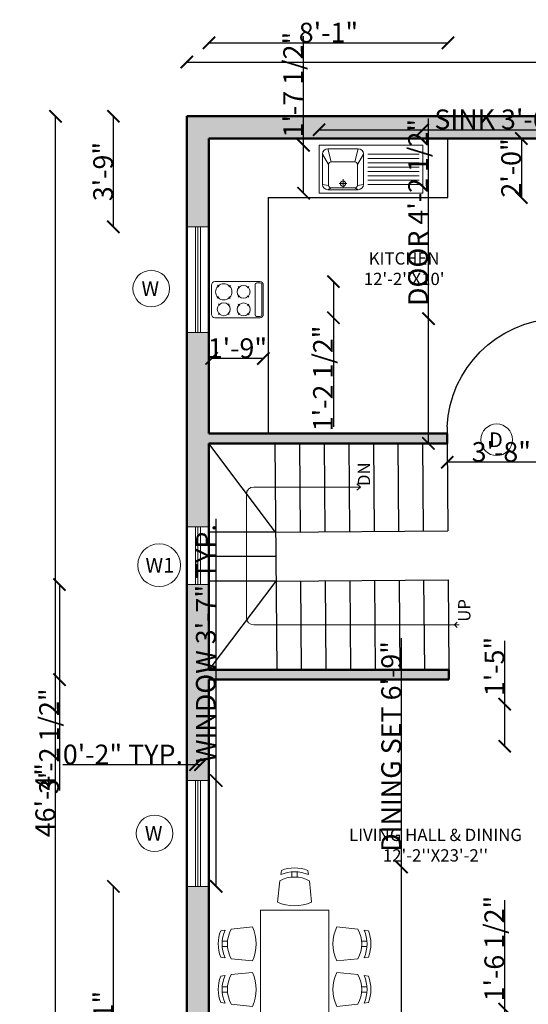
# Model space of a CAD drawing. Units: inches. Extents: x 2169 to 2662, y 1518 to 2151.
# Tile 4 of 6: x 2196 to 2403, y 1751 to 2151. Entities that reach past the tile are written whole.
import ezdxf

# ---------------------------------------------------------------- set-up
doc = ezdxf.new("R2010")
doc.units = ezdxf.units.IN
for name, color, linetype, lineweight in [('A-ANNO-DIMS', 2, 'Continuous', 18), ('A-ANNO-SYMB', 7, 'Continuous', 18), ('A-ANNO-TEXT', 7, 'Continuous', 18), ('A-AREA-IDEN', 7, 'Continuous', 18), ('A-EQPM', 8, 'Continuous', 18), ('A-FLOR-FIXT', 9, 'Continuous', 18), ('A-FURN', 8, 'Continuous', 18), ('A-WALL-PATT', 30, 'Continuous', 13), ('Doors', 240, 'Continuous', 30), ('Kitchen', 70, 'Continuous', 25), ('Steps', 50, 'Continuous', 25), ('Walls', 7, 'Continuous', 50), ('Windows', 160, 'Continuous', 18)]:
    doc.layers.add(name, color=color, linetype=linetype, lineweight=lineweight)
doc.styles.get("Standard").update_dxf_attribs({"font": 'arial.ttf'})
doc.dimstyles.get("Standard").update_dxf_attribs({"dimtxt": 8, "dimasz": 5, "dimexe": 0.18, "dimexo": 0.0625, "dimgap": 0.09, "dimtad": 1, "dimdec": 1, "dimzin": 0, "dimdsep": 46, "dimlunit": 4, "dimtxsty": 'Standard', "dimblk": 'ARCHTICK', "dimcen": 0.09, "dimse1": 1, "dimse2": 1, "dimadec": 0, "dimazin": 0, "dimtfac": 1, "dimtdec": 1, "dimtofl": 0, "dimtmove": 0, "dimatfit": 3, "dimfxl": 1, "dimtolj": 1, "dimtzin": 0, "dimarcsym": 0})

# ---------------------------------------------------------------- blocks, each defined once
blk = doc.blocks.new('_ArchTick')
at = {"color": 0, "linetype": 'ByBlock', "const_width": 0.15}
blk.add_lwpolyline([(-0.5, -0.5), (0.5, 0.5)], dxfattribs=at)
blk = doc.blocks.new('*D2')
at = {"layer": 'A-ANNO-DIMS', "color": 0, "lineweight": -2, "transparency": 16777216}
blk.add_line((2263.98, 2133.67), (2575.98, 2133.67), dxfattribs=at)
at = {"layer": 'Defpoints', "color": 0, "transparency": 16777216}
for p in [(2575.98, 2133.67), (2263.98, 2111.6), (2575.98, 2111.6)]:
    blk.add_point(p, dxfattribs=at)
at = {"layer": 'A-ANNO-DIMS', "color": 0, "lineweight": -2, "transparency": 16777216, "xscale": 5, "yscale": 5, "zscale": 5, "rotation": 180}
blk.add_blockref('_ArchTick', (2263.98, 2133.67), dxfattribs=at)
at = {"layer": 'A-ANNO-DIMS', "color": 0, "lineweight": -2, "transparency": 16777216, "xscale": 5, "yscale": 5, "zscale": 5}
blk.add_blockref('_ArchTick', (2575.98, 2133.67), dxfattribs=at)
at = {"layer": 'A-ANNO-DIMS', "color": 0, "transparency": 16777216, "insert": (2419.98, 2137.85), "char_height": 8, "attachment_point": 5}
blk.add_mtext("\\A1;26'", dxfattribs=at)
blk = doc.blocks.new('*D4')
at = {"layer": 'A-ANNO-DIMS', "color": 0, "lineweight": -2, "transparency": 16777216}
blk.add_line((2210.62, 1555.6), (2210.62, 2111.6), dxfattribs=at)
at = {"layer": 'Defpoints', "color": 0, "transparency": 16777216}
for p in [(2210.62, 2111.6), (2263.98, 2111.6), (2263.98, 1555.6)]:
    blk.add_point(p, dxfattribs=at)
at = {"layer": 'A-ANNO-DIMS', "color": 0, "lineweight": -2, "transparency": 16777216, "xscale": 5, "yscale": 5, "zscale": 5}
for p, rotation in [((2210.62, 2111.6), 90), ((2210.62, 1555.6), 270)]:
    blk.add_blockref('_ArchTick', p, dxfattribs=dict(at, rotation=rotation))
at = {"layer": 'A-ANNO-DIMS', "color": 0, "transparency": 16777216, "insert": (2206.45, 1833.6), "char_height": 8, "attachment_point": 5, "rotation": 90}
blk.add_mtext('\\A1;46\'-4"', dxfattribs=at)
blk = doc.blocks.new('table-23')
at = {"color": 0, "linetype": 'ByBlock'}
for p, q in [((-0.632, 0.469), (-0.624, 0.525)), ((-0.268, 0.469), (-0.276, 0.525)), ((-0.485, 0.506), (-0.485, 0.436)), ((-0.415, 0.506), (-0.415, 0.436)), ((-0.675, 0.107), (-0.645, 0.387)), ((-0.225, 0.107), (-0.255, 0.387)), ((-0.9, -1.492), (-0.9, 0)), ((-0.9, 0), (0, 0)), ((0, -1.492), (0, 0)), ((-1.006, -0.221), (-1.286, -0.251)), ((0.106, -0.221), (0.386, -0.251)), ((-1.368, -0.264), (-1.424, -0.273)), ((0.468, -0.264), (0.524, -0.273)), ((-1.405, -0.411), (-1.335, -0.411)), ((-1.405, -0.481), (-1.335, -0.481)), ((0.505, -0.411), (0.435, -0.411)), ((0.505, -0.481), (0.435, -0.481)), ((-1.368, -0.628), (-1.424, -0.62)), ((-1.006, -0.671), (-1.286, -0.641)), ((0.106, -0.671), (0.386, -0.641)), ((0.468, -0.628), (0.524, -0.62)), ((-1.368, -0.864), (-1.424, -0.873)), ((-1.006, -0.821), (-1.286, -0.851)), ((0.106, -0.821), (0.386, -0.851)), ((0.468, -0.864), (0.524, -0.873)), ((-1.405, -1.011), (-1.335, -1.011)), ((0.505, -1.011), (0.435, -1.011)), ((-1.405, -1.081), (-1.335, -1.081)), ((0.505, -1.081), (0.435, -1.081)), ((-1.368, -1.228), (-1.424, -1.22)), ((-1.006, -1.271), (-1.286, -1.241)), ((0.106, -1.271), (0.386, -1.241)), ((0.468, -1.228), (0.524, -1.22)), ((-0.9, -1.492), (0, -1.492)), ((-0.675, -1.599), (-0.645, -1.879)), ((-0.225, -1.599), (-0.255, -1.879)), ((-0.485, -1.998), (-0.485, -1.928)), ((-0.415, -1.998), (-0.415, -1.928)), ((-0.632, -1.961), (-0.624, -2.017)), ((-0.268, -1.961), (-0.276, -2.017))]:
    blk.add_line(p, q, dxfattribs=at)
for centre, radius, start, end in [((-0.45, 0.077), 0.48, 68.7887, 111.2113), ((-0.45, 0.032), 0.405, 61.2372, 118.7628), ((-0.45, 0.057), 0.45, 66.1344, 113.8656), ((-0.45, 0.588), 0.531, 244.9424, 295.0576), ((-0.931, -0.446), 0.405, 151.2372, 208.7628), ((-1.487, -0.446), 0.531, 334.9424, 25.0576), ((0.587, -0.446), 0.531, 154.9424, 205.0576), ((0.031, -0.446), 0.405, 331.2372, 28.7628), ((-0.977, -0.446), 0.48, 158.7887, 201.2113), ((-0.956, -0.446), 0.45, 156.1344, 203.8656), ((0.056, -0.446), 0.45, 336.1344, 23.8656), ((0.077, -0.446), 0.48, 338.7887, 21.2113), ((-0.977, -1.046), 0.48, 158.7887, 201.2113), ((-0.956, -1.046), 0.45, 156.1344, 203.8656), ((-0.931, -1.046), 0.405, 151.2372, 208.7628), ((-1.487, -1.046), 0.531, 334.9424, 25.0576), ((0.587, -1.046), 0.531, 154.9424, 205.0576), ((0.031, -1.046), 0.405, 331.2372, 28.7628), ((0.056, -1.046), 0.45, 336.1344, 23.8656), ((0.077, -1.046), 0.48, 338.7887, 21.2113), ((-0.45, -2.081), 0.531, 64.9424, 115.0576), ((-0.45, -1.524), 0.405, 241.2372, 298.7628), ((-0.45, -1.549), 0.45, 246.1344, 293.8656), ((-0.45, -1.57), 0.48, 248.7887, 291.2113)]:
    blk.add_arc(centre, radius, start, end, dxfattribs=at)
blk = doc.blocks.new('KK')
for p, q in [((0, 0.55), (0, 0)), ((1.19, 0.55), (0, 0.55)), ((0.1, 0.51), (0.14, 0.36)), ((0.45, 0.51), (0.1, 0.51)), ((0.41, 0.36), (0.45, 0.51)), ((1.19, 0), (1.19, 0.55)), ((0.11, 0.33), (0.04, 0.45)), ((0.04, 0.45), (0.04, 0.1)), ((0.14, 0.36), (0.41, 0.36)), ((0.44, 0.33), (0.51, 0.45)), ((0.51, 0.1), (0.51, 0.45)), ((0.56, 0.45), (1.15, 0.45)), ((0.56, 0.4), (1.15, 0.4)), ((0.56, 0.35), (1.15, 0.35)), ((0.11, 0.09), (0.11, 0.33)), ((0.44, 0.33), (0.44, 0.09)), ((0.56, 0.3), (1.15, 0.3)), ((0.56, 0.25), (1.15, 0.25)), ((0.275, 0.06), (0.275, 0.16)), ((0.56, 0.2), (1.15, 0.2)), ((0.56, 0.15), (1.15, 0.15)), ((0, 0), (1.19, 0)), ((0.04, 0.1), (0.11, 0.09)), ((0.14, 0.06), (0.1, 0.04)), ((0.1, 0.04), (0.45, 0.04)), ((0.41, 0.06), (0.14, 0.06)), ((0.23, 0.11), (0.32, 0.11)), ((0.41, 0.06), (0.45, 0.04)), ((0.44, 0.09), (0.51, 0.1)), ((0.56, 0.1), (1.15, 0.1))]:
    blk.add_line(p, q)
blk.add_circle((0.275, 0.11), 0.03)
for centre, radius, start, end in [((0.1, 0.45), 0.06, 90, 180), ((0.45, 0.45), 0.06, 0, 90), ((0.14, 0.33), 0.03, 90, 180), ((0.41, 0.33), 0.03, 0, 90), ((0.1, 0.1), 0.06, 180, 270), ((0.14, 0.09), 0.03, 180, 270), ((0.41, 0.09), 0.03, 270, 0), ((0.45, 0.1), 0.06, 270, 0)]:
    blk.add_arc(centre, radius, start, end)
blk = doc.blocks.new('AP0B05')
for p, q in [((35, 100), (35, 880)), ((75, 100), (75, 878.9)), ((35, 100), (35, -20)), ((815, 100), (815, -20))]:
    blk.add_line(p, q)
blk.add_lwpolyline([(35, 100), (75, 100)])
blk.add_arc((-2.4, 62.6), 818.3, 2.62122, 87.37878)
blk = doc.blocks.new('GLAZING-43IN')
for p, q in [((-21.5, 1), (21.5, 1)), ((-21.5, 0), (21.5, 0)), ((-21.5, -1), (21.5, -1))]:
    blk.add_line(p, q)
blk = doc.blocks.new('GLAZING-SHORT')
for p, q in [((-1, -11.72), (-1, 11.72)), ((0, -11.72), (0, 11.72)), ((1, -11.72), (1, 11.72))]:
    blk.add_line(p, q)
blk = doc.blocks.new('OPENING-TAG-W')
blk.add_circle((0, 0), 7.42)
blk.add_text('W', height=6).set_placement((-3.96, -3))
blk = doc.blocks.new('OPENING-TAG-D')
blk.add_circle((0, 0), 6.43)
blk.add_text('D', height=6).set_placement((-3.13, -3))
blk = doc.blocks.new('*D25')
at = {"layer": 'A-ANNO-DIMS', "color": 0, "lineweight": -2, "transparency": 16777216}
for p, q in [((2275.93, 1841.55), (2275.93, 1947.96)), ((2275.93, 1798.55), (2275.93, 1841.55))]:
    blk.add_line(p, q, dxfattribs=at)
at = {"layer": 'Defpoints', "color": 0, "transparency": 16777216}
for p in [(2269.48, 1841.55), (2275.93, 1841.55), (2269.48, 1798.55)]:
    blk.add_point(p, dxfattribs=at)
at = {"layer": 'A-ANNO-DIMS', "color": 0, "lineweight": -2, "transparency": 16777216, "xscale": 5, "yscale": 5, "zscale": 5}
for p, rotation in [((2275.93, 1841.55), 90), ((2275.93, 1798.55), 270)]:
    blk.add_blockref('_ArchTick', p, dxfattribs=dict(at, rotation=rotation))
at = {"layer": 'A-ANNO-DIMS', "color": 0, "transparency": 16777216, "insert": (2271.69, 1897.25), "char_height": 8, "attachment_point": 5, "rotation": 90}
blk.add_mtext('\\A1;WINDOW 3\'-7" TYP.', dxfattribs=at)
blk = doc.blocks.new('*D26')
at = {"layer": 'A-ANNO-DIMS', "color": 0, "lineweight": -2, "transparency": 16777216}
for p, q in [((2267.48, 1848), (2213.53, 1848)), ((2269.48, 1848), (2267.48, 1848))]:
    blk.add_line(p, q, dxfattribs=at)
at = {"layer": 'Defpoints', "color": 0, "transparency": 16777216}
for p in [(2267.48, 1848), (2267.48, 1841.55), (2269.48, 1841.55)]:
    blk.add_point(p, dxfattribs=at)
at = {"layer": 'A-ANNO-DIMS', "color": 0, "lineweight": -2, "transparency": 16777216, "xscale": 5, "yscale": 5, "zscale": 5, "rotation": 180}
blk.add_blockref('_ArchTick', (2267.48, 1848), dxfattribs=at)
at = {"layer": 'A-ANNO-DIMS', "color": 0, "lineweight": -2, "transparency": 16777216, "xscale": 5, "yscale": 5, "zscale": 5}
blk.add_blockref('_ArchTick', (2269.48, 1848), dxfattribs=at)
at = {"layer": 'A-ANNO-DIMS', "color": 0, "transparency": 16777216, "insert": (2238, 1852.17), "char_height": 8, "attachment_point": 5}
blk.add_mtext('\\A1;0\'-2" TYP.', dxfattribs=at)
blk = doc.blocks.new('*D31')
at = {"layer": 'A-ANNO-DIMS', "color": 0, "lineweight": -2, "transparency": 16777216}
for p, q in [((2362.16, 2029.35), (2362.16, 2110.67)), ((2362.16, 1978.6), (2362.16, 2029.35))]:
    blk.add_line(p, q, dxfattribs=at)
at = {"layer": 'Defpoints', "color": 0, "transparency": 16777216}
for p in [(2362.16, 2029.35), (2369.77, 2029.35), (2369.77, 1978.6)]:
    blk.add_point(p, dxfattribs=at)
at = {"layer": 'A-ANNO-DIMS', "color": 0, "lineweight": -2, "transparency": 16777216, "xscale": 5, "yscale": 5, "zscale": 5}
for p, rotation in [((2362.16, 2029.35), 90), ((2362.16, 1978.6), 270)]:
    blk.add_blockref('_ArchTick', p, dxfattribs=dict(at, rotation=rotation))
at = {"layer": 'A-ANNO-DIMS', "color": 0, "transparency": 16777216, "insert": (2357.93, 2072.51), "char_height": 8, "attachment_point": 5, "rotation": 90}
blk.add_mtext('\\A1;DOOR 4\'-2 1/2"', dxfattribs=at)
blk = doc.blocks.new('*D32')
at = {"layer": 'A-ANNO-DIMS', "color": 0, "lineweight": -2, "transparency": 16777216}
blk.add_line((2413.75, 1970.99), (2369.77, 1970.99), dxfattribs=at)
at = {"layer": 'Defpoints', "color": 0, "transparency": 16777216}
for p in [(2369.77, 1978.6), (2413.75, 1978.6), (2369.77, 1970.99)]:
    blk.add_point(p, dxfattribs=at)
at = {"layer": 'A-ANNO-DIMS', "color": 0, "lineweight": -2, "transparency": 16777216, "xscale": 5, "yscale": 5, "zscale": 5, "rotation": 180}
blk.add_blockref('_ArchTick', (2369.77, 1970.99), dxfattribs=at)
at = {"layer": 'A-ANNO-DIMS', "color": 0, "lineweight": -2, "transparency": 16777216, "xscale": 5, "yscale": 5, "zscale": 5}
blk.add_blockref('_ArchTick', (2413.75, 1970.99), dxfattribs=at)
at = {"layer": 'A-ANNO-DIMS', "color": 0, "transparency": 16777216, "insert": (2391.76, 1975.17), "char_height": 8, "attachment_point": 5}
blk.add_mtext('\\A1;3\'-8"', dxfattribs=at)
blk = doc.blocks.new('*D47')
at = {"layer": 'A-ANNO-DIMS', "color": 0, "lineweight": -2, "transparency": 16777216}
for p, q in [((2351.22, 1806.38), (2351.22, 1899.49)), ((2351.22, 1725.43), (2351.22, 1806.38))]:
    blk.add_line(p, q, dxfattribs=at)
at = {"layer": 'Defpoints', "color": 0, "transparency": 16777216}
for p in [(2339.08, 1806.38), (2351.22, 1806.38), (2339.08, 1725.43)]:
    blk.add_point(p, dxfattribs=at)
at = {"layer": 'A-ANNO-DIMS', "color": 0, "lineweight": -2, "transparency": 16777216, "xscale": 5, "yscale": 5, "zscale": 5}
for p, rotation in [((2351.22, 1806.38), 90), ((2351.22, 1725.43), 270)]:
    blk.add_blockref('_ArchTick', p, dxfattribs=dict(at, rotation=rotation))
at = {"layer": 'A-ANNO-DIMS', "color": 0, "transparency": 16777216, "insert": (2347, 1855.43), "char_height": 8, "attachment_point": 5, "rotation": 90}
blk.add_mtext('\\A1;DINING SET 6\'-9"', dxfattribs=at)
blk = doc.blocks.new('*D53')
at = {"layer": 'A-ANNO-DIMS', "color": 0, "lineweight": -2, "transparency": 16777216}
for p, q in [((2317.71, 2106.14), (2359.84, 2106.14)), ((2359.84, 2106.14), (2415.44, 2106.14))]:
    blk.add_line(p, q, dxfattribs=at)
at = {"layer": 'Defpoints', "color": 0, "transparency": 16777216}
for p in [(2359.84, 2106.14), (2317.71, 2099.82), (2359.84, 2099.82)]:
    blk.add_point(p, dxfattribs=at)
at = {"layer": 'A-ANNO-DIMS', "color": 0, "lineweight": -2, "transparency": 16777216, "xscale": 5, "yscale": 5, "zscale": 5, "rotation": 180}
blk.add_blockref('_ArchTick', (2317.71, 2106.14), dxfattribs=at)
at = {"layer": 'A-ANNO-DIMS', "color": 0, "lineweight": -2, "transparency": 16777216, "xscale": 5, "yscale": 5, "zscale": 5}
blk.add_blockref('_ArchTick', (2359.84, 2106.14), dxfattribs=at)
at = {"layer": 'A-ANNO-DIMS', "color": 0, "transparency": 16777216, "insert": (2390.14, 2110.37), "char_height": 8, "attachment_point": 5}
blk.add_mtext('\\A1;SINK 3\'-6"', dxfattribs=at)
blk = doc.blocks.new('*D54')
at = {"layer": 'A-ANNO-DIMS', "color": 0, "lineweight": -2, "transparency": 16777216}
for p, q in [((2311.39, 2099.82), (2311.39, 2144.15)), ((2311.39, 2080.34), (2311.39, 2099.82))]:
    blk.add_line(p, q, dxfattribs=at)
at = {"layer": 'Defpoints', "color": 0, "transparency": 16777216}
for p in [(2311.39, 2099.82), (2317.71, 2099.82), (2317.71, 2080.34)]:
    blk.add_point(p, dxfattribs=at)
at = {"layer": 'A-ANNO-DIMS', "color": 0, "lineweight": -2, "transparency": 16777216, "xscale": 5, "yscale": 5, "zscale": 5}
for p, rotation in [((2311.39, 2099.82), 90), ((2311.39, 2080.34), 270)]:
    blk.add_blockref('_ArchTick', p, dxfattribs=dict(at, rotation=rotation))
at = {"layer": 'A-ANNO-DIMS', "color": 0, "transparency": 16777216, "insert": (2307.16, 2124.48), "char_height": 8, "attachment_point": 5, "rotation": 90}
blk.add_mtext('\\A1;1\'-7 1/2"', dxfattribs=at)
blk = doc.blocks.new('*D59')
at = {"layer": 'A-ANNO-DIMS', "color": 0, "lineweight": -2, "transparency": 16777216}
blk.add_line((2234.13, 1689.49), (2234.13, 1798.55), dxfattribs=at)
at = {"layer": 'Defpoints', "color": 0, "transparency": 16777216}
for p in [(2234.13, 1798.55), (2263.98, 1798.55), (2263.98, 1689.49)]:
    blk.add_point(p, dxfattribs=at)
at = {"layer": 'A-ANNO-DIMS', "color": 0, "lineweight": -2, "transparency": 16777216, "xscale": 5, "yscale": 5, "zscale": 5}
for p, rotation in [((2234.13, 1798.55), 90), ((2234.13, 1689.49), 270)]:
    blk.add_blockref('_ArchTick', p, dxfattribs=dict(at, rotation=rotation))
at = {"layer": 'A-ANNO-DIMS', "color": 0, "transparency": 16777216, "insert": (2229.95, 1744.02), "char_height": 8, "attachment_point": 5, "rotation": 90}
blk.add_mtext('\\A1;9\'-1"', dxfattribs=at)
blk = doc.blocks.new('*D60')
at = {"layer": 'A-ANNO-DIMS', "color": 0, "lineweight": -2, "transparency": 16777216}
blk.add_line((2234.13, 2066.68), (2234.13, 2111.6), dxfattribs=at)
at = {"layer": 'Defpoints', "color": 0, "transparency": 16777216}
for p in [(2234.13, 2111.6), (2263.98, 2111.6), (2263.98, 2066.68)]:
    blk.add_point(p, dxfattribs=at)
at = {"layer": 'A-ANNO-DIMS', "color": 0, "lineweight": -2, "transparency": 16777216, "xscale": 5, "yscale": 5, "zscale": 5}
for p, rotation in [((2234.13, 2111.6), 90), ((2234.13, 2066.68), 270)]:
    blk.add_blockref('_ArchTick', p, dxfattribs=dict(at, rotation=rotation))
at = {"layer": 'A-ANNO-DIMS', "color": 0, "transparency": 16777216, "insert": (2229.95, 2089.14), "char_height": 8, "attachment_point": 5, "rotation": 90}
blk.add_mtext('\\A1;3\'-9"', dxfattribs=at)
blk = doc.blocks.new('*D68')
at = {"layer": 'A-ANNO-DIMS', "color": 0, "lineweight": -2, "transparency": 16777216}
blk.add_line((2272.98, 2141.45), (2370.07, 2141.45), dxfattribs=at)
at = {"layer": 'Defpoints', "color": 0, "transparency": 16777216}
for p in [(2370.07, 2141.45), (2272.98, 2102.6), (2370.07, 2102.6)]:
    blk.add_point(p, dxfattribs=at)
at = {"layer": 'A-ANNO-DIMS', "color": 0, "lineweight": -2, "transparency": 16777216, "xscale": 5, "yscale": 5, "zscale": 5, "rotation": 180}
blk.add_blockref('_ArchTick', (2272.98, 2141.45), dxfattribs=at)
at = {"layer": 'A-ANNO-DIMS', "color": 0, "lineweight": -2, "transparency": 16777216, "xscale": 5, "yscale": 5, "zscale": 5}
blk.add_blockref('_ArchTick', (2370.07, 2141.45), dxfattribs=at)
at = {"layer": 'A-ANNO-DIMS', "color": 0, "transparency": 16777216, "insert": (2321.52, 2145.63), "char_height": 8, "attachment_point": 5}
blk.add_mtext('\\A1;8\'-1"', dxfattribs=at)
blk = doc.blocks.new('*D69')
at = {"layer": 'A-ANNO-DIMS', "color": 0, "lineweight": -2, "transparency": 16777216}
blk.add_line((2399.92, 2102.6), (2399.92, 2078.6), dxfattribs=at)
at = {"layer": 'Defpoints', "color": 0, "transparency": 16777216}
for p in [(2370.07, 2102.6), (2370.07, 2078.6), (2399.92, 2078.6)]:
    blk.add_point(p, dxfattribs=at)
at = {"layer": 'A-ANNO-DIMS', "color": 0, "lineweight": -2, "transparency": 16777216, "xscale": 5, "yscale": 5, "zscale": 5}
for p, rotation in [((2399.92, 2102.6), 90), ((2399.92, 2078.6), 270)]:
    blk.add_blockref('_ArchTick', p, dxfattribs=dict(at, rotation=rotation))
at = {"layer": 'A-ANNO-DIMS', "color": 0, "transparency": 16777216, "insert": (2395.74, 2090.6), "char_height": 8, "attachment_point": 5, "rotation": 90}
blk.add_mtext('\\A1;2\'-0"', dxfattribs=at)
blk = doc.blocks.new('*D70')
at = {"layer": 'A-ANNO-DIMS', "color": 0, "lineweight": -2, "transparency": 16777216}
blk.add_line((2272.98, 1525.75), (2370.48, 1525.75), dxfattribs=at)
at = {"layer": 'Defpoints', "color": 0, "transparency": 16777216}
for p in [(2272.98, 1886.6), (2370.48, 1886.6), (2370.48, 1525.75)]:
    blk.add_point(p, dxfattribs=at)
at = {"layer": 'A-ANNO-DIMS', "color": 0, "lineweight": -2, "transparency": 16777216, "xscale": 5, "yscale": 5, "zscale": 5, "rotation": 180}
blk.add_blockref('_ArchTick', (2272.98, 1525.75), dxfattribs=at)
at = {"layer": 'A-ANNO-DIMS', "color": 0, "lineweight": -2, "transparency": 16777216, "xscale": 5, "yscale": 5, "zscale": 5}
blk.add_blockref('_ArchTick', (2370.48, 1525.75), dxfattribs=at)
at = {"layer": 'A-ANNO-DIMS', "color": 0, "transparency": 16777216, "insert": (2321.73, 1529.98), "char_height": 8, "attachment_point": 5}
blk.add_mtext('\\A1;8\'-1 1/2"', dxfattribs=at)
blk = doc.blocks.new('*D71')
at = {"layer": 'A-ANNO-DIMS', "color": 0, "lineweight": -2, "transparency": 16777216}
for p, q in [((2300.48, 1525.75), (2310.48, 1525.75)), ((2310.48, 1525.75), (2343.14, 1525.75))]:
    blk.add_line(p, q, dxfattribs=at)
at = {"layer": 'Defpoints', "color": 0, "transparency": 16777216}
for p in [(2300.48, 1886.6), (2310.48, 1886.6), (2310.48, 1525.75)]:
    blk.add_point(p, dxfattribs=at)
at = {"layer": 'A-ANNO-DIMS', "color": 0, "lineweight": -2, "transparency": 16777216, "xscale": 5, "yscale": 5, "zscale": 5, "rotation": 180}
blk.add_blockref('_ArchTick', (2300.48, 1525.75), dxfattribs=at)
at = {"layer": 'A-ANNO-DIMS', "color": 0, "lineweight": -2, "transparency": 16777216, "xscale": 5, "yscale": 5, "zscale": 5}
blk.add_blockref('_ArchTick', (2310.48, 1525.75), dxfattribs=at)
at = {"layer": 'A-ANNO-DIMS', "color": 0, "transparency": 16777216, "insert": (2329.31, 1529.93), "char_height": 8, "attachment_point": 5}
blk.add_mtext('\\A1;0\'-10"', dxfattribs=at)
blk = doc.blocks.new('*D72')
at = {"layer": 'A-ANNO-DIMS', "color": 0, "lineweight": -2, "transparency": 16777216}
blk.add_line((2624.02, 1978.6), (2624.02, 1942.6), dxfattribs=at)
at = {"layer": 'Defpoints', "color": 0, "transparency": 16777216}
for p in [(2299.77, 1978.6), (2300.05, 1942.6), (2624.02, 1942.6)]:
    blk.add_point(p, dxfattribs=at)
at = {"layer": 'A-ANNO-DIMS', "color": 0, "lineweight": -2, "transparency": 16777216, "xscale": 5, "yscale": 5, "zscale": 5}
for p, rotation in [((2624.02, 1978.6), 90), ((2624.02, 1942.6), 270)]:
    blk.add_blockref('_ArchTick', p, dxfattribs=dict(at, rotation=rotation))
at = {"layer": 'A-ANNO-DIMS', "color": 0, "transparency": 16777216, "insert": (2619.84, 1960.6), "char_height": 8, "attachment_point": 5, "rotation": 90}
blk.add_mtext('\\A1;3\'-0"', dxfattribs=at)
blk = doc.blocks.new('*D73')
at = {"layer": 'A-ANNO-DIMS', "color": 0, "lineweight": -2, "transparency": 16777216}
blk.add_line((2624.02, 1886.6), (2624.02, 1978.6), dxfattribs=at)
at = {"layer": 'Defpoints', "color": 0, "transparency": 16777216}
for p in [(2369.77, 1978.6), (2624.02, 1978.6), (2370.48, 1886.6)]:
    blk.add_point(p, dxfattribs=at)
at = {"layer": 'A-ANNO-DIMS', "color": 0, "lineweight": -2, "transparency": 16777216, "xscale": 5, "yscale": 5, "zscale": 5}
for p, rotation in [((2624.02, 1978.6), 90), ((2624.02, 1886.6), 270)]:
    blk.add_blockref('_ArchTick', p, dxfattribs=dict(at, rotation=rotation))
at = {"layer": 'A-ANNO-DIMS', "color": 0, "transparency": 16777216, "insert": (2619.84, 1932.6), "char_height": 8, "attachment_point": 5, "rotation": 90}
blk.add_mtext('\\A1;7\'-8"', dxfattribs=at)
blk = doc.blocks.new('*D74')
at = {"layer": 'A-ANNO-DIMS', "color": 0, "lineweight": -2, "transparency": 16777216}
for p, q in [((2272.98, 1525.75), (2300.48, 1525.75)), ((2300.48, 1525.75), (2345.7, 1525.75))]:
    blk.add_line(p, q, dxfattribs=at)
at = {"layer": 'Defpoints', "color": 0, "transparency": 16777216}
for p in [(2272.98, 1886.6), (2300.48, 1886.6), (2300.48, 1525.75)]:
    blk.add_point(p, dxfattribs=at)
at = {"layer": 'A-ANNO-DIMS', "color": 0, "lineweight": -2, "transparency": 16777216, "xscale": 5, "yscale": 5, "zscale": 5, "rotation": 180}
blk.add_blockref('_ArchTick', (2272.98, 1525.75), dxfattribs=at)
at = {"layer": 'A-ANNO-DIMS', "color": 0, "lineweight": -2, "transparency": 16777216, "xscale": 5, "yscale": 5, "zscale": 5}
blk.add_blockref('_ArchTick', (2300.48, 1525.75), dxfattribs=at)
at = {"layer": 'A-ANNO-DIMS', "color": 0, "transparency": 16777216, "insert": (2325.59, 1529.98), "char_height": 8, "attachment_point": 5}
blk.add_mtext('\\A1;2\'-3 1/2"', dxfattribs=at)
blk = doc.blocks.new('*D75')
at = {"layer": 'A-ANNO-DIMS', "color": 0, "lineweight": -2, "transparency": 16777216}
for p, q in [((2212.23, 1921.26), (2212.23, 1882.6)), ((2212.23, 1882.6), (2212.23, 1837.52))]:
    blk.add_line(p, q, dxfattribs=at)
at = {"layer": 'Defpoints', "color": 0, "transparency": 16777216}
for p in [(2263.98, 1921.26), (2212.23, 1882.6), (2272.98, 1882.6)]:
    blk.add_point(p, dxfattribs=at)
at = {"layer": 'A-ANNO-DIMS', "color": 0, "lineweight": -2, "transparency": 16777216, "xscale": 5, "yscale": 5, "zscale": 5}
for p, rotation in [((2212.23, 1921.26), 90), ((2212.23, 1882.6), 270)]:
    blk.add_blockref('_ArchTick', p, dxfattribs=dict(at, rotation=rotation))
at = {"layer": 'A-ANNO-DIMS', "color": 0, "transparency": 16777216, "insert": (2208, 1857.56), "char_height": 8, "attachment_point": 5, "rotation": 90}
blk.add_mtext('\\A1;3\'-2 1/2"', dxfattribs=at)
blk = doc.blocks.new('*D78')
at = {"layer": 'A-ANNO-DIMS', "color": 0, "lineweight": -2, "transparency": 16777216}
for p, q in [((2393.13, 1748.6), (2393.13, 1792.94)), ((2393.13, 1729.93), (2393.13, 1748.6))]:
    blk.add_line(p, q, dxfattribs=at)
at = {"layer": 'Defpoints', "color": 0, "transparency": 16777216}
for p in [(2393.13, 1748.6), (2422.98, 1748.6), (2422.98, 1729.93)]:
    blk.add_point(p, dxfattribs=at)
at = {"layer": 'A-ANNO-DIMS', "color": 0, "lineweight": -2, "transparency": 16777216, "xscale": 5, "yscale": 5, "zscale": 5}
for p, rotation in [((2393.13, 1748.6), 90), ((2393.13, 1729.93), 270)]:
    blk.add_blockref('_ArchTick', p, dxfattribs=dict(at, rotation=rotation))
at = {"layer": 'A-ANNO-DIMS', "color": 0, "transparency": 16777216, "insert": (2388.9, 1773.27), "char_height": 8, "attachment_point": 5, "rotation": 90}
blk.add_mtext('\\A1;1\'-6 1/2"', dxfattribs=at)
blk = doc.blocks.new('*D79')
at = {"layer": 'A-ANNO-DIMS', "color": 0, "lineweight": -2, "transparency": 16777216}
for p, q in [((2393.13, 1872.6), (2393.13, 1898.3)), ((2393.13, 1855.49), (2393.13, 1872.6))]:
    blk.add_line(p, q, dxfattribs=at)
at = {"layer": 'Defpoints', "color": 0, "transparency": 16777216}
for p in [(2393.13, 1872.6), (2422.98, 1872.6), (2422.98, 1855.49)]:
    blk.add_point(p, dxfattribs=at)
at = {"layer": 'A-ANNO-DIMS', "color": 0, "lineweight": -2, "transparency": 16777216, "xscale": 5, "yscale": 5, "zscale": 5}
for p, rotation in [((2393.13, 1872.6), 90), ((2393.13, 1855.49), 270)]:
    blk.add_blockref('_ArchTick', p, dxfattribs=dict(at, rotation=rotation))
at = {"layer": 'A-ANNO-DIMS', "color": 0, "transparency": 16777216, "insert": (2388.95, 1887.95), "char_height": 8, "attachment_point": 5, "rotation": 90}
blk.add_mtext('\\A1;1\'-5"', dxfattribs=at)
blk = doc.blocks.new('*D82')
at = {"layer": 'A-ANNO-DIMS', "color": 0, "lineweight": -2, "transparency": 16777216}
blk.add_line((2295.05, 2013.16), (2274.01, 2013.16), dxfattribs=at)
at = {"layer": 'Defpoints', "color": 0, "transparency": 16777216}
for p in [(2274.01, 2043.01), (2295.05, 2043.01), (2274.01, 2013.16)]:
    blk.add_point(p, dxfattribs=at)
at = {"layer": 'A-ANNO-DIMS', "color": 0, "lineweight": -2, "transparency": 16777216, "xscale": 5, "yscale": 5, "zscale": 5, "rotation": 180}
blk.add_blockref('_ArchTick', (2274.01, 2013.16), dxfattribs=at)
at = {"layer": 'A-ANNO-DIMS', "color": 0, "lineweight": -2, "transparency": 16777216, "xscale": 5, "yscale": 5, "zscale": 5}
blk.add_blockref('_ArchTick', (2295.05, 2013.16), dxfattribs=at)
at = {"layer": 'A-ANNO-DIMS', "color": 0, "transparency": 16777216, "insert": (2284.53, 2017.33), "char_height": 8, "attachment_point": 5}
blk.add_mtext('\\A1;1\'-9"', dxfattribs=at)
blk = doc.blocks.new('*D83')
at = {"layer": 'A-ANNO-DIMS', "color": 0, "lineweight": -2, "transparency": 16777216}
for p, q in [((2323.52, 2044.39), (2323.52, 2029.72)), ((2323.52, 2029.72), (2323.52, 1985.38))]:
    blk.add_line(p, q, dxfattribs=at)
at = {"layer": 'Defpoints', "color": 0, "transparency": 16777216}
for p in [(2293.67, 2044.39), (2293.67, 2029.72), (2323.52, 2029.72)]:
    blk.add_point(p, dxfattribs=at)
at = {"layer": 'A-ANNO-DIMS', "color": 0, "lineweight": -2, "transparency": 16777216, "xscale": 5, "yscale": 5, "zscale": 5}
for p, rotation in [((2323.52, 2044.39), 90), ((2323.52, 2029.72), 270)]:
    blk.add_blockref('_ArchTick', p, dxfattribs=dict(at, rotation=rotation))
at = {"layer": 'A-ANNO-DIMS', "color": 0, "transparency": 16777216, "insert": (2319.29, 2005.05), "char_height": 8, "attachment_point": 5, "rotation": 90}
blk.add_mtext('\\A1;1\'-2 1/2"', dxfattribs=at)

msp = doc.modelspace()

# ---------------------------------------------------------------- hatches: boundary and pattern name
at = {"layer": 'A-WALL-PATT', "transparency": 33554585}
h = msp.add_hatch(color=256, dxfattribs=at)
h.dxf.hatch_style = 1
h.paths.add_polyline_path([(2575.98, 2111.6), (2263.98, 2111.6), (2263.98, 2066.68), (2272.98, 2066.68), (2272.98, 2102.6), (2418.98, 2102.6), (2418.98, 1982.6), (2413.75, 1982.6), (2413.75, 1978.6), (2418.98, 1978.6), (2418.98, 1954.6), (2429.26, 1954.6), (2429.26, 1958.6), (2422.98, 1958.6), (2422.98, 2102.6), (2566.98, 2102.6), (2566.98, 2052.1), (2575.98, 2052.1)])
h.paths.add_polyline_path([(2575.98, 2009.1), (2566.98, 2009.1), (2566.98, 1997.84), (2566.98, 1958.6), (2467.98, 1958.6), (2467.98, 1950.67), (2471.98, 1950.67), (2471.98, 1954.6), (2566.98, 1954.6), (2566.98, 1947.83), (2575.98, 1947.83)])
h.paths.add_polyline_path([(2272.98, 2023.68), (2263.98, 2023.68), (2263.98, 1944.7), (2272.98, 1944.7), (2272.98, 1978.6), (2369.77, 1978.6), (2369.77, 1982.6), (2272.98, 1982.6)])
h.paths.add_polyline_path([(2272.98, 1882.6), (2370.48, 1882.6), (2370.48, 1886.6), (2272.98, 1886.6), (2272.98, 1921.26), (2263.98, 1921.26), (2263.98, 1841.55), (2272.98, 1841.55)])
h.paths.add_polyline_path([(2272.98, 1798.55), (2263.98, 1798.55), (2263.98, 1689.49), (2272.98, 1689.49)])
h.paths.add_polyline_path([(2272.98, 1646.49), (2263.98, 1646.49), (2263.98, 1595.6), (2281.85, 1595.6), (2281.85, 1604.6), (2272.98, 1604.6)])
h.paths.add_polyline_path([(2342.72, 1600.02), (2342.72, 1604.6), (2324.85, 1604.6), (2324.85, 1595.6), (2342.72, 1595.6)])
h.paths.add_polyline_path([(2462.45, 1604.6), (2408.92, 1604.6), (2408.92, 1595.6), (2462.45, 1595.6)])
h.paths.add_polyline_path([(2422.98, 1689.75), (2418.98, 1689.75), (2418.98, 1604.6), (2422.98, 1604.6)])
h.paths.add_polyline_path([(2575.98, 1655.1), (2566.98, 1655.1), (2566.98, 1643.84), (2566.98, 1604.6), (2522.45, 1604.6), (2522.45, 1595.6), (2575.98, 1595.6)])
h.paths.add_polyline_path([(2575.98, 1791.1), (2566.98, 1791.1), (2566.98, 1752.6), (2422.98, 1752.6), (2422.98, 1816.31), (2418.98, 1816.31), (2418.98, 1729.93), (2422.98, 1729.93), (2422.98, 1748.6), (2566.98, 1748.6), (2566.98, 1698.1), (2575.98, 1698.1)])
h.paths.add_polyline_path([(2575.98, 1883.38), (2566.98, 1883.38), (2566.98, 1876.6), (2506.75, 1876.6), (2506.75, 1872.6), (2566.98, 1872.6), (2566.98, 1834.1), (2575.98, 1834.1)])
h.paths.add_polyline_path([(2477.81, 1876.6), (2471.98, 1876.6), (2471.98, 1913.6), (2566.98, 1913.6), (2566.98, 1906.83), (2575.98, 1906.83), (2575.98, 1924.38), (2566.98, 1924.38), (2566.98, 1917.6), (2471.98, 1917.6), (2471.98, 1921.14), (2467.98, 1921.14), (2467.98, 1876.6), (2418.98, 1876.6), (2418.98, 1855.49), (2422.98, 1855.49), (2422.98, 1872.6), (2477.81, 1872.6)])

# ---------------------------------------------------------------- linework, layer by layer
at = {"layer": 'A-ANNO-SYMB'}
for p, q in [((2334.55, 1960.87), (2333, 1962.2)), ((2288.18, 1907.87), (2288.18, 1957.87)), ((2334.55, 1960.87), (2291.18, 1960.87)), ((2334.55, 1960.87), (2333, 1959.55)), ((2372.67, 1904.87), (2373.78, 1905.92)), ((2374.58, 1904.87), (2291.18, 1904.87)), ((2372.67, 1904.87), (2373.78, 1903.83))]:
    msp.add_line(p, q, dxfattribs=at)
msp.add_circle((2252.73, 1929.12), 8.72, dxfattribs=at)
for centre, start, end in [((2291.18, 1957.87), 90, 180), ((2291.18, 1907.87), 180, 270)]:
    msp.add_arc(centre, 3, start, end, dxfattribs=at)
at = {"layer": 'A-EQPM'}
for p, q in [((2274.01, 2043.01), (2274.01, 2031.1)), ((2293.67, 2044.39), (2275.39, 2044.39)), ((2276.39, 2042.93), (2277, 2042.28)), ((2281.69, 2042.84), (2281.04, 2042.23)), ((2284.83, 2042.4), (2285.42, 2041.82)), ((2289.18, 2042.42), (2288.6, 2041.84)), ((2291.73, 2043.28), (2291.73, 2030.82)), ((2293.67, 2043.84), (2292.28, 2043.84)), ((2294.5, 2031.1), (2294.5, 2043.01)), ((2295.05, 2031.1), (2295.05, 2043.01)), ((2276.3, 2037.64), (2276.95, 2038.25)), ((2281.59, 2037.54), (2280.98, 2038.19)), ((2284.86, 2038.05), (2285.44, 2038.64)), ((2289.21, 2038.08), (2288.62, 2038.65)), ((2276.8, 2035.33), (2277.39, 2034.78)), ((2281.14, 2035.37), (2280.59, 2034.78)), ((2284.87, 2035.23), (2285.46, 2034.68)), ((2289.21, 2035.27), (2288.66, 2034.68)), ((2275.39, 2029.72), (2293.67, 2029.72)), ((2276.84, 2030.99), (2277.39, 2031.57)), ((2281.18, 2031.03), (2280.6, 2031.58)), ((2284.91, 2030.89), (2285.46, 2031.48)), ((2289.25, 2030.93), (2288.67, 2031.48)), ((2292.28, 2030.27), (2293.67, 2030.27))]:
    msp.add_line(p, q, dxfattribs=at)
for centre, radius, start, end in [((2275.39, 2043.01), 1.38, 90, 180), ((2278.99, 2040.24), 3.3, 138.017, 221.983), ((2278.99, 2040.24), 3.3, 48.017, 131.983), ((2278.99, 2040.24), 3.3, 318.017, 41.983), ((2287.02, 2040.24), 2.63, 138.017, 221.983), ((2287.02, 2040.24), 2.63, 48.017, 131.983), ((2287.02, 2040.24), 2.63, 318.017, 41.983), ((2292.28, 2043.28), 0.554, 90, 180), ((2293.67, 2043.01), 1.38, 0, 90), ((2293.67, 2043.01), 0.831, 0, 90), ((2278.99, 2040.24), 3.3, 228.017, 311.983), ((2287.02, 2040.24), 2.63, 228.017, 311.983), ((2278.99, 2033.18), 2.63, 138.017, 221.983), ((2278.99, 2033.18), 2.63, 48.017, 131.983), ((2278.99, 2033.18), 2.63, 318.017, 41.983), ((2287.06, 2033.08), 2.63, 138.017, 221.983), ((2287.06, 2033.08), 2.63, 48.017, 131.983), ((2287.06, 2033.08), 2.63, 318.017, 41.983), ((2275.39, 2031.1), 1.38, 180, 270), ((2278.99, 2033.18), 2.63, 228.017, 311.983), ((2287.06, 2033.08), 2.63, 228.017, 311.983), ((2292.28, 2030.82), 0.554, 180, 270), ((2293.67, 2031.1), 1.38, 270, 0), ((2293.67, 2031.1), 0.831, 270, 0)]:
    msp.add_arc(centre, radius, start, end, dxfattribs=at)
at = {"layer": 'Kitchen'}
for p, q in [((2370.07, 2078.6), (2370.07, 2102.6)), ((2296.98, 2078.6), (2370.07, 2078.6)), ((2296.98, 2078.6), (2296.98, 1982.6))]:
    msp.add_line(p, q, dxfattribs=at)
at = {"layer": 'Steps'}
for p, q in [((2300.05, 1942.6), (2272.98, 1978.6)), ((2299.77, 1978.6), (2300.48, 1886.6)), ((2309.77, 1978.6), (2310.04, 1942.68)), ((2319.77, 1978.6), (2320.04, 1942.76)), ((2329.77, 1978.6), (2330.04, 1942.84)), ((2339.77, 1978.6), (2340.04, 1942.91)), ((2349.77, 1978.6), (2350.04, 1942.99)), ((2359.77, 1978.6), (2360.04, 1943.07)), ((2369.77, 1978.6), (2370.04, 1943.14)), ((2300.12, 1942.6), (2272.98, 1942.6)), ((2300.05, 1942.6), (2370.04, 1943.14)), ((2300.12, 1932.6), (2272.98, 1932.6)), ((2300.12, 1922.6), (2272.98, 1922.6)), ((2300.12, 1922.6), (2272.98, 1886.6)), ((2300.12, 1922.6), (2370.2, 1923.14)), ((2310.2, 1922.68), (2310.48, 1886.6)), ((2320.2, 1922.76), (2320.48, 1886.6)), ((2330.2, 1922.84), (2330.48, 1886.6)), ((2340.2, 1922.91), (2340.48, 1886.6)), ((2350.2, 1922.99), (2350.48, 1886.6)), ((2360.2, 1923.07), (2360.48, 1886.6)), ((2370.2, 1923.14), (2370.48, 1886.6))]:
    msp.add_line(p, q, dxfattribs=at)
at = {"layer": 'Walls'}
for p, q in [((2263.98, 2111.6), (2575.98, 2111.6)), ((2263.98, 2111.6), (2263.98, 1555.6)), ((2272.98, 2102.6), (2418.98, 2102.6)), ((2272.98, 2102.6), (2272.98, 1982.6)), ((2272.98, 1982.6), (2369.77, 1982.6)), ((2369.77, 1978.6), (2369.77, 1982.6)), ((2272.98, 1978.6), (2369.77, 1978.6)), ((2272.98, 1978.6), (2272.98, 1886.6)), ((2272.98, 1886.6), (2370.48, 1886.6)), ((2370.48, 1886.6), (2370.48, 1882.6)), ((2272.98, 1882.6), (2370.48, 1882.6)), ((2272.98, 1882.6), (2272.98, 1604.6))]:
    msp.add_line(p, q, dxfattribs=at)
at = {"layer": 'Windows'}
for points in [[(2263.98, 2023.68), (2263.98, 2066.68), (2272.98, 2066.68), (2272.98, 2023.68)], [(2263.98, 1921.26), (2263.98, 1944.7), (2272.98, 1944.7), (2272.98, 1921.26)], [(2263.98, 1798.55), (2263.98, 1841.55), (2272.98, 1841.55), (2272.98, 1798.55)]]:
    msp.add_lwpolyline(points, close=True, dxfattribs=at)

# ---------------------------------------------------------------- block references
at = {"layer": 'A-ANNO-SYMB'}
for name, p in [('OPENING-TAG-W', (2249.49, 2041.58)), ('OPENING-TAG-D', (2389.87, 1980.1)), ('OPENING-TAG-W', (2250.85, 1820.1))]:
    msp.add_blockref(name, p, dxfattribs=at)
at = {"layer": 'A-FLOR-FIXT', "xscale": 35.40674051187821, "yscale": 35.40674051187821, "zscale": 35.40674051187821}
msp.add_blockref('KK', (2317.71, 2080.34), dxfattribs=at)
at = {"layer": 'A-FURN', "xscale": 30.80298432698044, "yscale": 30.80298432698044, "zscale": 30.80298432698044}
msp.add_blockref('table-23', (2321.61, 1788.89), dxfattribs=at)
at = {"layer": 'Doors', "xscale": -0.0563843061810126, "yscale": 0.0563843061810126, "zscale": 0.0563843061810126}
msp.add_blockref('AP0B05', (2415.72, 1979.73), dxfattribs=at)
at = {"layer": 'Windows', "rotation": 89.99999999999991}
for p in [(2268.48, 2045.18), (2268.48, 1820.05)]:
    msp.add_blockref('GLAZING-43IN', p, dxfattribs=at)
at = {"layer": 'Windows'}
msp.add_blockref('GLAZING-SHORT', (2268.48, 1932.98), dxfattribs=at)

# ---------------------------------------------------------------- texts
at = {"layer": 'A-ANNO-SYMB'}
msp.add_text('W1', height=6, dxfattribs=at).set_placement((2247.16, 1926.1))
at = {"layer": 'A-ANNO-TEXT', "char_height": 5, "attachment_point": 1, "rotation": 90}
for s, insert in [('\\pxqc;DN', (2333.45, 1958.69)), ('\\pxqc;UP', (2374.22, 1903.33))]:
    msp.add_mtext_dynamic_manual_height_columns(s, width=14.813, gutter_width=12.5, heights=[0], dxfattribs=dict(at, insert=insert))
at = {"layer": 'A-AREA-IDEN', "char_height": 5, "attachment_point": 1}
for s, width, heights, insert in [("\\pxqc;KITCHEN\\P12'-2''X10'", 63.1797, [0], (2320.68, 2056.32)), ("\\pxqc;LIVING HALL & DINING\\P12'-2''X23'-2''", 84.4317, [21.95], (2322.8, 1821.98))]:
    msp.add_mtext_dynamic_manual_height_columns(s, width=width, gutter_width=12.5, heights=heights, dxfattribs=dict(at, insert=insert))

# ---------------------------------------------------------------- dimensions: what is measured, and where the dimension line sits
at = {"layer": 'A-ANNO-DIMS'}
for base, p1, p2, override, picture, middle in [((2370.07, 2141.45), (2272.98, 2102.6), (2370.07, 2102.6), {"dimdec": 1, "dimlfac": 1, "dimrnd": 0, "dimzin": 1, "dimdsep": 46, "dimlunit": 4, "dimfrac": 2}, '*D68', (2321.52, 2145.63)), ((2575.98, 2133.67), (2263.98, 2111.6), (2575.98, 2111.6), {"dimclrd": 0, "dimclre": 0, "dimclrt": 0}, '*D2', (2419.98, 2137.85)), ((2370.48, 1525.75), (2272.98, 1886.6), (2370.48, 1886.6), {"dimdec": 1, "dimlfac": 1, "dimrnd": 0, "dimzin": 1, "dimdsep": 46, "dimlunit": 4, "dimfrac": 2}, '*D70', (2321.73, 1529.98)), ((2300.48, 1525.75), (2272.98, 1886.6), (2300.48, 1886.6), {"dimdec": 1, "dimlfac": 1, "dimrnd": 0, "dimzin": 1, "dimdsep": 46, "dimlunit": 4, "dimfrac": 2}, '*D74', (2325.59, 1529.98)), ((2310.48, 1525.75), (2300.48, 1886.6), (2310.48, 1886.6), {"dimdec": 1, "dimlfac": 1, "dimrnd": 0, "dimzin": 1, "dimdsep": 46, "dimlunit": 4, "dimfrac": 2}, '*D71', (2329.31, 1529.93))]:
    dim = msp.add_linear_dim(base=base, p1=p1, p2=p2, dimstyle='Standard', override=override, dxfattribs=at)
    dim.commit()
    dim.dimension.update_dxf_attribs({"geometry": picture, "text_midpoint": middle})
for base, p1, p2, angle, override, picture, middle in [((2311.39, 2099.82), (2317.71, 2080.34), (2317.71, 2099.82), 90, {"dimdec": 1, "dimlfac": 1, "dimrnd": 0, "dimzin": 1, "dimdsep": 46, "dimlunit": 4, "dimfrac": 2}, '*D54', (2307.16, 2124.48)), ((2210.62, 2111.6), (2263.98, 1555.6), (2263.98, 2111.6), 90, {"dimclrd": 0, "dimclre": 0, "dimclrt": 0}, '*D4', (2206.45, 1833.6)), ((2234.13, 2111.6), (2263.98, 2066.68), (2263.98, 2111.6), 90, {"dimdec": 1, "dimlfac": 1, "dimrnd": 0, "dimzin": 1, "dimdsep": 46, "dimlunit": 4, "dimfrac": 2}, '*D60', (2229.95, 2089.14)), ((2399.92, 2078.6), (2370.07, 2102.6), (2370.07, 2078.6), 270, {"dimdec": 1, "dimlfac": 1, "dimrnd": 0, "dimzin": 1, "dimdsep": 46, "dimlunit": 4, "dimfrac": 2}, '*D69', (2395.74, 2090.6)), ((2323.52, 2029.72), (2293.67, 2044.39), (2293.67, 2029.72), 270, {"dimdec": 1, "dimlfac": 1, "dimrnd": 0, "dimzin": 1, "dimdsep": 46, "dimlunit": 4, "dimfrac": 2}, '*D83', (2319.29, 2005.05)), ((2274.01, 2013.16), (2295.05, 2043.01), (2274.01, 2043.01), 180, {"dimdec": 1, "dimlfac": 1, "dimrnd": 0, "dimzin": 1, "dimdsep": 46, "dimlunit": 4, "dimfrac": 2}, '*D82', (2284.53, 2017.33)), ((2624.02, 1942.6), (2299.77, 1978.6), (2300.05, 1942.6), 90, {"dimdec": 1, "dimlfac": 1, "dimrnd": 0, "dimzin": 1, "dimdsep": 46, "dimlunit": 4, "dimfrac": 2}, '*D72', (2619.84, 1960.6)), ((2624.02, 1978.6), (2370.48, 1886.6), (2369.77, 1978.6), 90, {"dimdec": 1, "dimlfac": 1, "dimrnd": 0, "dimzin": 1, "dimdsep": 46, "dimlunit": 4, "dimfrac": 2}, '*D73', (2619.84, 1932.6)), ((2369.77, 1970.99), (2413.75, 1978.6), (2369.77, 1978.6), 180, {"dimdec": 1, "dimlfac": 1, "dimrnd": 0, "dimzin": 1, "dimdsep": 46, "dimlunit": 4, "dimfrac": 2}, '*D32', (2391.76, 1975.17)), ((2212.23, 1882.6), (2263.98, 1921.26), (2272.98, 1882.6), 90, {"dimdec": 1, "dimlfac": 1, "dimrnd": 0, "dimzin": 1, "dimdsep": 46, "dimlunit": 4, "dimfrac": 2}, '*D75', (2208, 1857.56)), ((2393.13, 1872.6), (2422.98, 1855.49), (2422.98, 1872.6), 90, {"dimdec": 1, "dimlfac": 1, "dimrnd": 0, "dimzin": 1, "dimdsep": 46, "dimlunit": 4, "dimfrac": 2}, '*D79', (2388.95, 1887.95)), ((2234.13, 1798.55), (2263.98, 1689.49), (2263.98, 1798.55), 90, {"dimdec": 1, "dimlfac": 1, "dimrnd": 0, "dimzin": 1, "dimdsep": 46, "dimlunit": 4, "dimfrac": 2}, '*D59', (2229.95, 1744.02)), ((2393.13, 1748.6), (2422.98, 1729.93), (2422.98, 1748.6), 90, {"dimdec": 1, "dimlfac": 1, "dimrnd": 0, "dimzin": 1, "dimdsep": 46, "dimlunit": 4, "dimfrac": 2}, '*D78', (2388.9, 1773.27))]:
    dim = msp.add_linear_dim(base=base, p1=p1, p2=p2, angle=angle, dimstyle='Standard', override=override, dxfattribs=at)
    dim.commit()
    dim.dimension.update_dxf_attribs({"geometry": picture, "text_midpoint": middle})
dim = msp.add_linear_dim(base=(2359.84, 2106.14), p1=(2317.71, 2099.82), p2=(2359.84, 2099.82), text='SINK <>', dimstyle='Standard', override={"dimdec": 1, "dimlfac": 1, "dimrnd": 0, "dimzin": 1, "dimdsep": 46, "dimlunit": 4, "dimfrac": 2}, dxfattribs=at)
dim.commit()
dim.dimension.update_dxf_attribs({"geometry": '*D53', "text_midpoint": (2390.14, 2110.37)})
for base, p1, p2, angle, text, picture, middle in [((2362.1569, 2029.3504), (2369.7688, 1978.6045), (2369.7688, 2029.3504), 90, 'DOOR <>', '*D31', (2357.9278, 2072.5114)), ((2275.93, 1841.55), (2269.48, 1798.55), (2269.48, 1841.55), 90, 'WINDOW <> TYP.', '*D25', (2271.69, 1897.25)), ((2351.2225, 1806.38), (2339.0798, 1725.4288), (2339.0798, 1806.38), 90, 'DINING SET <>', '*D47', (2346.9961, 1855.4345)), ((2267.48, 1848), (2269.48, 1841.55), (2267.48, 1841.55), 180, '<> TYP.', '*D26', (2238, 1852.17))]:
    dim = msp.add_linear_dim(base=base, p1=p1, p2=p2, angle=angle, text=text, dimstyle='Standard', override={"dimdec": 1, "dimlfac": 1, "dimrnd": 0, "dimzin": 1, "dimdsep": 46, "dimlunit": 4, "dimfrac": 2}, dxfattribs=at)
    dim.commit()
    dim.dimension.update_dxf_attribs({"geometry": picture, "text_midpoint": middle})

doc.saveas('drawing.dxf')
